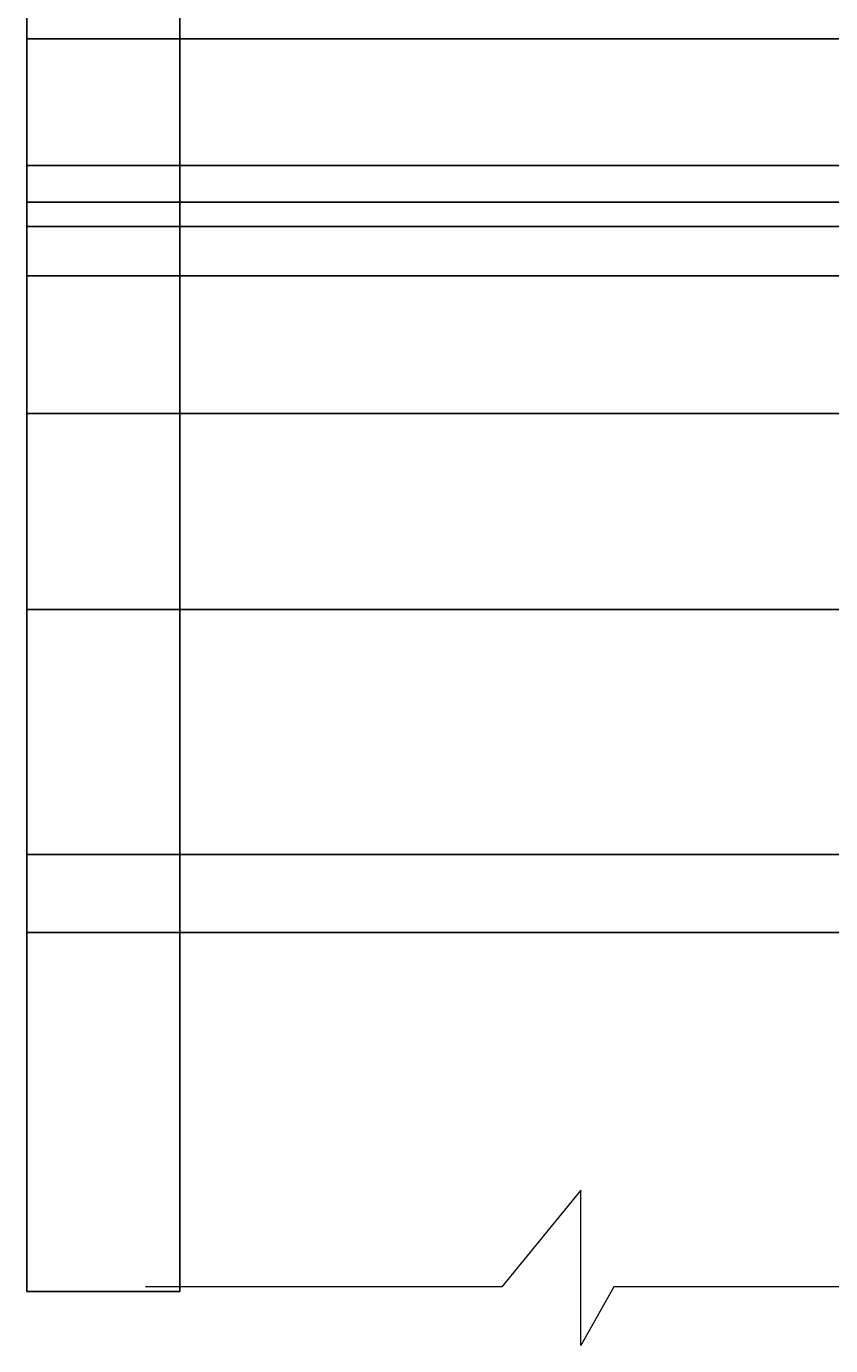
# Model space of a CAD drawing. Units: inches. Extents: x 154617 to 156384, y 250671 to 252576.
# Tile 1 of 6: x 154617 to 155207, y 250758 to 251728. Entities that reach past the tile are written whole.
import ezdxf

# ---------------------------------------------------------------- set-up
doc = ezdxf.new("R2010")
doc.units = ezdxf.units.IN
for name, color, linetype, lineweight in [('A-ANNO-DIMS', 2, 'Continuous', 18), ('C-ANNO-BRKL', 7, 'Continuous', 18), ('C-ROAD', 7, 'Continuous', 25)]:
    doc.layers.add(name, color=color, linetype=linetype, lineweight=lineweight)
doc.styles.get("Standard").update_dxf_attribs({"font": 'arial.ttf'})
doc.dimstyles.get("Standard").update_dxf_attribs({"dimtxt": 0.18, "dimasz": 0.18, "dimexe": 0.18, "dimexo": 0.0625, "dimgap": 0.09, "dimtad": 0, "dimtih": 1, "dimtoh": 1, "dimdec": 4, "dimzin": 0, "dimdsep": 46, "dimtxsty": 'Standard', "dimcen": 0.09, "dimadec": 0, "dimazin": 0, "dimtfac": 1, "dimtdec": 4, "dimtofl": 0, "dimtmove": 0, "dimatfit": 3, "dimfxl": 1, "dimtolj": 1, "dimtzin": 0, "dimarcsym": 0})

# ---------------------------------------------------------------- blocks, each defined once
blk = doc.blocks.new('ROAD-BREAK')
for p, q in [((319.88, 114.19), (261.89, 43.25)), ((319.88, 0), (319.88, 114.19)), ((261.89, 43.25), (0, 43.25)), ((344.19, 43.25), (319.88, 0)), ((540.36, 43.25), (344.19, 43.25))]:
    blk.add_line(p, q)
blk = doc.blocks.new('*D23')
at = {"layer": 'A-ANNO-DIMS', "color": 0, "lineweight": -2, "transparency": 16777216}
for p, q in [((154729.17, 252414.5), (154616.73, 252414.5)), ((154616.91, 252414.32), (154616.91, 251606.56)), ((154616.91, 250798.45), (154616.91, 251606.2)), ((154729.17, 250798.27), (154616.73, 250798.27))]:
    blk.add_line(p, q, dxfattribs=at)
at = {"layer": 'A-ANNO-DIMS', "color": 0, "transparency": 16777216}
for points in [[(154616.88, 252414.32), (154616.94, 252414.32), (154616.91, 252414.5)], [(154616.88, 250798.45), (154616.94, 250798.45), (154616.91, 250798.27)]]:
    blk.add_solid(points, dxfattribs=at)
at = {"layer": 'Defpoints', "color": 0, "transparency": 16777216}
for p in [(154616.91, 252414.5), (154729.24, 252414.5), (154729.24, 250798.27)]:
    blk.add_point(p, dxfattribs=at)
at = {"layer": 'A-ANNO-DIMS', "color": 0, "transparency": 16777216, "insert": (154616.91, 251606.38), "char_height": 0.18, "attachment_point": 5}
blk.add_mtext('\\A1;1616.2', dxfattribs=at)
blk = doc.blocks.new('*D30')
at = {"layer": 'A-ANNO-DIMS', "color": 0, "lineweight": -2, "transparency": 16777216}
for p, q in [((155324.78, 251581.16), (154616.73, 251581.16)), ((154616.91, 251580.98), (154616.91, 251512.53)), ((154616.91, 251443.71), (154616.91, 251512.16)), ((155324.78, 251443.53), (154616.73, 251443.53))]:
    blk.add_line(p, q, dxfattribs=at)
at = {"layer": 'A-ANNO-DIMS', "color": 0, "transparency": 16777216}
for points in [[(154616.88, 251580.98), (154616.94, 251580.98), (154616.91, 251581.16)], [(154616.88, 251443.71), (154616.94, 251443.71), (154616.91, 251443.53)]]:
    blk.add_solid(points, dxfattribs=at)
at = {"layer": 'Defpoints', "color": 0, "transparency": 16777216}
for p in [(154616.91, 251581.16), (155324.84, 251581.16), (155324.84, 251443.53)]:
    blk.add_point(p, dxfattribs=at)
at = {"layer": 'A-ANNO-DIMS', "color": 0, "transparency": 16777216, "insert": (154616.91, 251512.35), "char_height": 0.18, "attachment_point": 5}
blk.add_mtext('\\A1;137.64', dxfattribs=at)
blk = doc.blocks.new('*D31')
at = {"layer": 'A-ANNO-DIMS', "color": 0, "lineweight": -2, "transparency": 16777216}
for p, q in [((155324.78, 251719.03), (154616.73, 251719.03)), ((154616.91, 251718.85), (154616.91, 251650.28)), ((154616.91, 251581.34), (154616.91, 251649.91)), ((155324.78, 251581.16), (154616.73, 251581.16))]:
    blk.add_line(p, q, dxfattribs=at)
at = {"layer": 'A-ANNO-DIMS', "color": 0, "transparency": 16777216}
for points in [[(154616.88, 251718.85), (154616.94, 251718.85), (154616.91, 251719.03)], [(154616.88, 251581.34), (154616.94, 251581.34), (154616.91, 251581.16)]]:
    blk.add_solid(points, dxfattribs=at)
at = {"layer": 'Defpoints', "color": 0, "transparency": 16777216}
for p in [(154616.91, 251719.03), (155324.84, 251719.03), (155324.84, 251581.16)]:
    blk.add_point(p, dxfattribs=at)
at = {"layer": 'A-ANNO-DIMS', "color": 0, "transparency": 16777216, "insert": (154616.91, 251650.1), "char_height": 0.18, "attachment_point": 5}
blk.add_mtext('\\A1;137.86', dxfattribs=at)
blk = doc.blocks.new('*D32')
at = {"layer": 'A-ANNO-DIMS', "color": 0, "lineweight": -2, "transparency": 16777216}
for p, q in [((155324.78, 251873.03), (154616.73, 251873.03)), ((154616.91, 251872.85), (154616.91, 251796.21)), ((154616.91, 251719.21), (154616.91, 251795.84)), ((155324.78, 251719.03), (154616.73, 251719.03))]:
    blk.add_line(p, q, dxfattribs=at)
at = {"layer": 'A-ANNO-DIMS', "color": 0, "transparency": 16777216}
for points in [[(154616.88, 251872.85), (154616.94, 251872.85), (154616.91, 251873.03)], [(154616.88, 251719.21), (154616.94, 251719.21), (154616.91, 251719.03)]]:
    blk.add_solid(points, dxfattribs=at)
at = {"layer": 'Defpoints', "color": 0, "transparency": 16777216}
for p in [(154616.91, 251873.03), (155324.84, 251873.03), (155324.84, 251719.03)]:
    blk.add_point(p, dxfattribs=at)
at = {"layer": 'A-ANNO-DIMS', "color": 0, "transparency": 16777216, "insert": (154616.91, 251796.03), "char_height": 0.18, "attachment_point": 5}
blk.add_mtext('\\A1;154', dxfattribs=at)
blk = doc.blocks.new('*D33')
at = {"layer": 'A-ANNO-DIMS', "color": 0, "lineweight": -2, "transparency": 16777216}
for p, q in [((155324.78, 251443.53), (154616.73, 251443.53)), ((154616.91, 251443.35), (154616.91, 251371.71)), ((154616.91, 251299.71), (154616.91, 251371.35)), ((155324.78, 251299.53), (154616.73, 251299.53))]:
    blk.add_line(p, q, dxfattribs=at)
at = {"layer": 'A-ANNO-DIMS', "color": 0, "transparency": 16777216}
for points in [[(154616.88, 251443.35), (154616.94, 251443.35), (154616.91, 251443.53)], [(154616.88, 251299.71), (154616.94, 251299.71), (154616.91, 251299.53)]]:
    blk.add_solid(points, dxfattribs=at)
at = {"layer": 'Defpoints', "color": 0, "transparency": 16777216}
for p in [(154616.91, 251443.53), (155324.84, 251443.53), (155324.84, 251299.53)]:
    blk.add_point(p, dxfattribs=at)
at = {"layer": 'A-ANNO-DIMS', "color": 0, "transparency": 16777216, "insert": (154616.91, 251371.53), "char_height": 0.18, "attachment_point": 5}
blk.add_mtext('\\A1;144', dxfattribs=at)
blk = doc.blocks.new('*D34')
at = {"layer": 'A-ANNO-DIMS', "color": 0, "lineweight": -2, "transparency": 16777216}
for p, q in [((155324.78, 251299.53), (154616.73, 251299.53)), ((154616.91, 251299.35), (154616.91, 251209.71)), ((154616.91, 251119.71), (154616.91, 251209.34)), ((155324, 251119.53), (154616.73, 251119.53))]:
    blk.add_line(p, q, dxfattribs=at)
at = {"layer": 'A-ANNO-DIMS', "color": 0, "transparency": 16777216}
for points in [[(154616.88, 251299.35), (154616.94, 251299.35), (154616.91, 251299.53)], [(154616.88, 251119.71), (154616.94, 251119.71), (154616.91, 251119.53)]]:
    blk.add_solid(points, dxfattribs=at)
at = {"layer": 'Defpoints', "color": 0, "transparency": 16777216}
for p in [(154616.91, 251299.53), (155324.84, 251299.53), (155324.06, 251119.53)]:
    blk.add_point(p, dxfattribs=at)
at = {"layer": 'A-ANNO-DIMS', "color": 0, "transparency": 16777216, "insert": (154616.91, 251209.53), "char_height": 0.18, "attachment_point": 5}
blk.add_mtext('\\A1;180', dxfattribs=at)
blk = doc.blocks.new('*D35')
at = {"layer": 'A-ANNO-DIMS', "color": 0, "lineweight": -2, "transparency": 16777216}
for p, q in [((155262.03, 251119.53), (154616.73, 251119.53)), ((154616.91, 251119.35), (154616.91, 251090.96)), ((154616.91, 251062.21), (154616.91, 251090.59)), ((155262.03, 251062.03), (154616.73, 251062.03))]:
    blk.add_line(p, q, dxfattribs=at)
at = {"layer": 'A-ANNO-DIMS', "color": 0, "transparency": 16777216}
for points in [[(154616.88, 251119.35), (154616.94, 251119.35), (154616.91, 251119.53)], [(154616.88, 251062.21), (154616.94, 251062.21), (154616.91, 251062.03)]]:
    blk.add_solid(points, dxfattribs=at)
at = {"layer": 'Defpoints', "color": 0, "transparency": 16777216}
for p in [(154616.91, 251119.53), (155262.1, 251119.53), (155262.1, 251062.03)]:
    blk.add_point(p, dxfattribs=at)
at = {"layer": 'A-ANNO-DIMS', "color": 0, "transparency": 16777216, "insert": (154616.91, 251090.78), "char_height": 0.18, "attachment_point": 5}
blk.add_mtext('\\A1;57.5', dxfattribs=at)
blk = doc.blocks.new('*D55')
at = {"layer": 'A-ANNO-DIMS', "color": 0, "lineweight": -2, "transparency": 16777216}
for p, q in [((155844.53, 251625.8), (154616.73, 251625.8)), ((154616.91, 251625.62), (154616.91, 251585.48)), ((154616.91, 251544.98), (154616.91, 251585.12)), ((155844.53, 251544.8), (154616.73, 251544.8))]:
    blk.add_line(p, q, dxfattribs=at)
at = {"layer": 'A-ANNO-DIMS', "color": 0, "transparency": 16777216}
for points in [[(154616.88, 251625.62), (154616.94, 251625.62), (154616.91, 251625.8)], [(154616.88, 251544.98), (154616.94, 251544.98), (154616.91, 251544.8)]]:
    blk.add_solid(points, dxfattribs=at)
at = {"layer": 'Defpoints', "color": 0, "transparency": 16777216}
for p in [(154616.91, 251625.8), (155844.6, 251625.8), (155844.6, 251544.8)]:
    blk.add_point(p, dxfattribs=at)
at = {"layer": 'A-ANNO-DIMS', "color": 0, "transparency": 16777216, "insert": (154616.91, 251585.3), "char_height": 0.18, "attachment_point": 5}
blk.add_mtext('\\A1;81', dxfattribs=at)
blk = doc.blocks.new('*D62')
at = {"layer": 'A-ANNO-DIMS', "color": 0, "lineweight": -2, "transparency": 16777216}
for p, q in [((155348.92, 251719.03), (154616.73, 251719.03)), ((154616.91, 251718.85), (154616.91, 251659.21)), ((154616.91, 251599.21), (154616.91, 251658.84)), ((155348.92, 251599.03), (154616.73, 251599.03))]:
    blk.add_line(p, q, dxfattribs=at)
at = {"layer": 'A-ANNO-DIMS', "color": 0, "transparency": 16777216}
for points in [[(154616.88, 251718.85), (154616.94, 251718.85), (154616.91, 251719.03)], [(154616.88, 251599.21), (154616.94, 251599.21), (154616.91, 251599.03)]]:
    blk.add_solid(points, dxfattribs=at)
at = {"layer": 'Defpoints', "color": 0, "transparency": 16777216}
for p in [(154616.91, 251719.03), (155348.98, 251719.03), (155348.98, 251599.03)]:
    blk.add_point(p, dxfattribs=at)
at = {"layer": 'A-ANNO-DIMS', "color": 0, "transparency": 16777216, "insert": (154616.91, 251659.03), "char_height": 0.18, "attachment_point": 5}
blk.add_mtext('\\A1;120', dxfattribs=at)

msp = doc.modelspace()

# ---------------------------------------------------------------- linework, layer by layer
at = {"layer": 'C-ROAD'}
msp.add_line((154729.237, 252414.495), (154729.237, 250798.266), dxfattribs=at)

# ---------------------------------------------------------------- block references
at = {"layer": 'C-ANNO-BRKL'}
msp.add_blockref('ROAD-BREAK', (154704.015, 250758.479), dxfattribs=at)

# ---------------------------------------------------------------- dimensions: what is measured, and where the dimension line sits
at = {"layer": 'A-ANNO-DIMS'}
for base, p1, p2, override, picture, middle in [((154616.915, 252414.495), (154729.237, 250798.266), (154729.237, 252414.495), {"dimdec": 1, "dimlfac": 1, "dimrnd": 0, "dimzin": 0, "dimdsep": 46, "dimlunit": 2}, '*D23', (154616.915, 251606.381)), ((154616.915, 251873.026), (155324.842, 251719.026), (155324.842, 251873.026), {"dimdec": 0, "dimlfac": 1, "dimrnd": 0, "dimzin": 0, "dimdsep": 46, "dimlunit": 2}, '*D32', (154616.915, 251796.026)), ((154616.915, 251719.026), (155324.842, 251581.164), (155324.842, 251719.026), {"dimdec": 2, "dimlfac": 1, "dimrnd": 0, "dimzin": 0, "dimdsep": 46, "dimlunit": 2}, '*D31', (154616.915, 251650.095)), ((154616.915, 251719.026), (155348.982, 251599.026), (155348.982, 251719.026), {"dimdec": 0, "dimlfac": 1, "dimrnd": 0, "dimzin": 0, "dimdsep": 46, "dimlunit": 2}, '*D62', (154616.915, 251659.026)), ((154616.915, 251625.802), (155844.597, 251544.802), (155844.597, 251625.802), {"dimdec": 0, "dimlfac": 1, "dimrnd": 0, "dimzin": 0, "dimdsep": 46, "dimlunit": 2}, '*D55', (154616.915, 251585.302)), ((154616.915, 251581.164), (155324.842, 251443.526), (155324.842, 251581.164), {"dimdec": 2, "dimlfac": 1, "dimrnd": 0, "dimzin": 0, "dimdsep": 46, "dimlunit": 2}, '*D30', (154616.915, 251512.345)), ((154616.915, 251443.526), (155324.842, 251299.526), (155324.842, 251443.526), {"dimdec": 0, "dimlfac": 1, "dimrnd": 0, "dimzin": 0, "dimdsep": 46, "dimlunit": 2}, '*D33', (154616.915, 251371.526)), ((154616.915, 251299.526), (155324.063, 251119.526), (155324.842, 251299.526), {"dimdec": 0, "dimlfac": 1, "dimrnd": 0, "dimzin": 0, "dimdsep": 46, "dimlunit": 2}, '*D34', (154616.915, 251209.526)), ((154616.915, 251119.526), (155262.097, 251062.026), (155262.097, 251119.526), {"dimdec": 1, "dimlfac": 1, "dimrnd": 0, "dimzin": 0, "dimdsep": 46, "dimlunit": 2}, '*D35', (154616.915, 251090.776))]:
    dim = msp.add_linear_dim(base=base, p1=p1, p2=p2, angle=90, dimstyle='Standard', override=override, dxfattribs=at)
    dim.commit()
    dim.dimension.update_dxf_attribs({"geometry": picture, "text_midpoint": middle})

doc.saveas('drawing.dxf')
